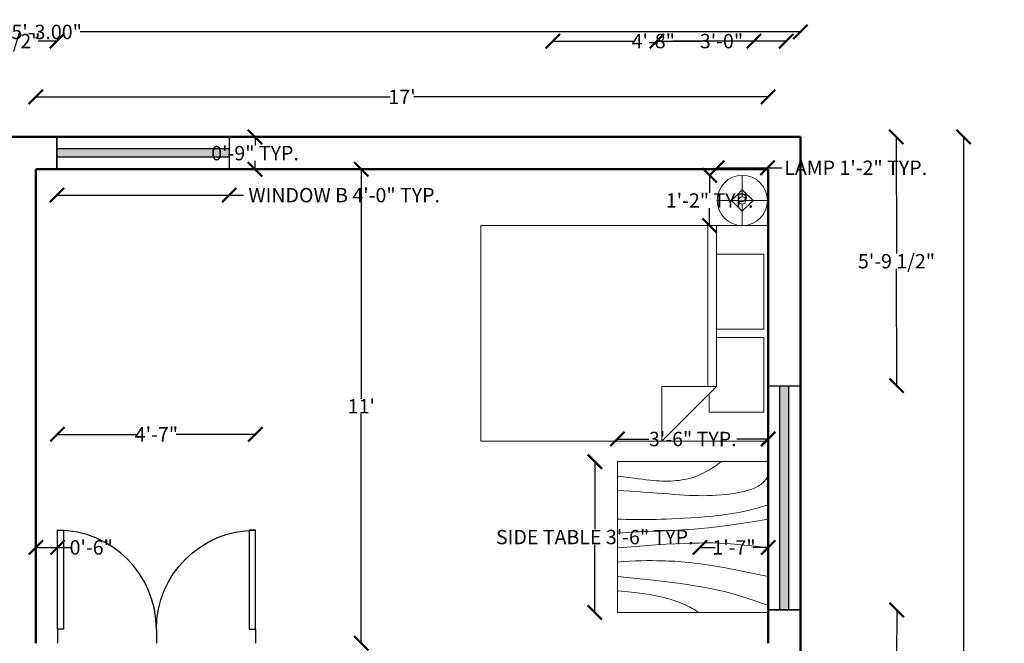
# Model space of a CAD drawing. Units: inches. Extents: x 2466 to 2986, y -30 to 527.
# Tile 5 of 5: x 2711 to 2986, y 354 to 527. Entities that reach past the tile are written whole.
import ezdxf

# ---------------------------------------------------------------- set-up
doc = ezdxf.new("R2010")
doc.units = ezdxf.units.IN
for name, color, linetype, lineweight in [('A-ANNO-DIMS', 2, 'Continuous', 18), ('A-GLAZ', 4, 'Continuous', 25), ('doors', 3, 'Continuous', 25), ('furniture', 6, 'Continuous', 18), ('walls', 40, 'Continuous', 50)]:
    doc.layers.add(name, color=color, linetype=linetype, lineweight=lineweight)
doc.styles.get("Standard").update_dxf_attribs({"font": 'arial.ttf'})
doc.dimstyles.get("Standard").update_dxf_attribs({"dimtxt": 4, "dimasz": 4, "dimexe": 0.18, "dimexo": 0.0625, "dimgap": 0.09, "dimtad": 0, "dimtih": 1, "dimtoh": 1, "dimzin": 0, "dimdsep": 46, "dimlunit": 3, "dimtxsty": 'Standard', "dimblk": 'ARCHTICK', "dimcen": 0.09, "dimse1": 1, "dimse2": 1, "dimclrd": 3, "dimclrt": 2, "dimadec": 0, "dimazin": 0, "dimtfac": 1, "dimtofl": 0, "dimtmove": 0, "dimatfit": 3, "dimfxl": 1, "dimtolj": 1, "dimtzin": 0, "dimarcsym": 0})

# ---------------------------------------------------------------- blocks, each defined once
blk = doc.blocks.new('*U8')
for p, q in [((0, 0), (0, -100)), ((700, 0), (700, -100))]:
    blk.add_line(p, q)
blk.add_lwpolyline([(0, 0), (0, 700), (43.75, 700), (43.75, 0)], close=True)
blk.add_arc((0, 0), 700, 0, 90)
blk = doc.blocks.new('Bed - Queen')
for p, q in [((0, -80.00003), (0, 0)), ((0, 0), (59.99999, 0)), ((59.99999, 0), (59.99999, -80.00003)), ((7.99999, -1.2), (28.79998, -1.2)), ((7.99999, -14.4), (7.99999, -1.2)), ((28.79998, -1.2), (28.79998, -14.4)), ((31.19999, -1.2), (51.99999, -1.2)), ((31.19999, -14.4), (31.19999, -1.2)), ((51.99999, -1.2), (51.99999, -16.4)), ((0, -14.4), (44.8, -14.4)), ((59.99999, -29.6), (44.8, -14.4)), ((44.8, -14.4), (44.8, -29.6)), ((51.99999, -16.4), (46.79936, -16.4)), ((44.8, -16.8), (0, -16.8)), ((44.8, -29.6), (59.99999, -29.6)), ((59.99999, -80.00003), (0, -80.00003))]:
    blk.add_line(p, q)
blk = doc.blocks.new('Lamp - Table')
for p, q in [((0, 7), (0, 1)), ((0, 3), (-3, 0)), ((3, 0), (0, 3)), ((-1, 0), (-7, 0)), ((-3, 0), (0, -3)), ((0, -3), (3, 0)), ((1, 0), (7, 0)), ((0, -1), (0, -7))]:
    blk.add_line(p, q)
for radius in [7, 1]:
    blk.add_circle((0, 0), radius)
blk = doc.blocks.new('Table - Square Woodgrain 42 x 42 in.')
blk.add_line((0, -42), (42, -42))
for points in [[(0, -4), (1.704, -4.2172), (3.2358, -4.4188), (4.615, -4.604), (5.8615, -4.7721), (6.9951, -4.9224), (8.0357, -5.0541), (9.0031, -5.1667), (9.9171, -5.2594), (10.7951, -5.3316), (11.6445, -5.3836), (12.4702, -5.4157), (13.277, -5.4283), (14.0698, -5.4217), (14.8535, -5.3964), (15.6331, -5.3526), (16.4133, -5.2908), (17.1986, -5.2103), (17.9913, -5.1062), (18.793, -4.9727), (19.6056, -4.8038), (20.4307, -4.5937), (21.2701, -4.3365), (22.1256, -4.0262), (22.9989, -3.6571), (23.888, -3.2272), (24.7756, -2.7516), (25.6408, -2.2491), (26.4624, -1.7387), (27.2195, -1.2395), (27.891, -0.7703), (28.456, -0.3501), (28.8934, 0.002)], [(0, -42), (0, 0), (42, 0), (42, -42)], [(0, -8), (1.8203, -8.1001), (3.6741, -8.2149), (5.5411, -8.3408), (7.4011, -8.4741), (9.2339, -8.6112), (11.0193, -8.7484), (12.7371, -8.8821), (14.3671, -9.0086), (15.8954, -9.1246), (17.3337, -9.2278), (18.6997, -9.3159), (20.0116, -9.387), (21.2871, -9.4389), (22.5442, -9.4696), (23.8008, -9.477), (25.0749, -9.459), (26.3791, -9.4137), (27.7049, -9.3403), (29.0383, -9.2382), (30.3655, -9.1068), (31.6728, -8.9455), (32.9461, -8.7535), (34.1717, -8.5304), (35.3358, -8.2756), (36.4268, -7.9863), (37.443, -7.6521), (38.3849, -7.2603), (39.253, -6.7986), (40.048, -6.2542), (40.7705, -5.6147), (41.421, -4.8674), (42, -4)], [(42, -12), (39.1784, -12.8621), (36.4519, -13.5654), (33.8246, -14.1294), (31.3004, -14.5731), (28.8832, -14.9161), (26.577, -15.1775), (24.3858, -15.3768), (22.3136, -15.5332), (20.3622, -15.6632), (18.5254, -15.7718), (16.7947, -15.8612), (15.1618, -15.9338), (13.6183, -15.9916), (12.1558, -16.0369), (10.7659, -16.0718), (9.4403, -16.0987), (8.1703, -16.1191), (6.9461, -16.1325), (5.7577, -16.1377), (4.595, -16.1335), (3.4479, -16.1188), (2.3064, -16.0924), (1.1604, -16.0532), (0, -16)], [(42, -16), (37.6529, -16.7365), (33.8802, -17.329), (30.6179, -17.7961), (27.8015, -18.1561), (25.3668, -18.4275), (23.2497, -18.6288), (21.3859, -18.7785), (19.7111, -18.8949), (18.1693, -18.9939), (16.7375, -19.0795), (15.401, -19.1534), (14.1449, -19.217), (12.9544, -19.2717), (11.8148, -19.3191), (10.7113, -19.3606), (9.6291, -19.3976), (8.5534, -19.4323), (7.47, -19.4689), (6.3643, -19.5122), (5.222, -19.5672), (4.0288, -19.6386), (2.7703, -19.7313), (1.4321, -19.8501), (0, -20)], [(0, -24), (3.9243, -23.6805), (7.4766, -23.4138), (10.6891, -23.1954), (13.5943, -23.0205), (16.2247, -22.8847), (18.6125, -22.7832), (20.7903, -22.7116), (22.7903, -22.6651), (24.6563, -22.642), (26.4764, -22.6507), (28.35, -22.7024), (30.3766, -22.8084), (32.6555, -22.98), (35.2861, -23.2283), (38.3678, -23.5645), (42, -24)], [(42, -32), (37.392, -31.017), (33.4585, -30.2231), (30.1291, -29.5949), (27.3334, -29.109), (25.0009, -28.742), (23.0612, -28.4707), (21.4439, -28.2716), (20.0786, -28.1215), (18.8998, -28.0002), (17.8609, -27.9014), (16.9206, -27.8219), (16.0371, -27.7588), (15.1691, -27.709), (14.2748, -27.6693), (13.3128, -27.6368), (12.2415, -27.6083), (11.0295, -27.5824), (9.6867, -27.5643), (8.233, -27.5608), (6.6884, -27.5787), (5.0728, -27.6248), (3.4062, -27.7058), (1.7086, -27.8286), (0, -28)], [(0, -32), (5.4026, -32.5358), (9.9494, -33.019), (13.7424, -33.4553), (16.8834, -33.8505), (19.4743, -34.2106), (21.6171, -34.5413), (23.4136, -34.8486), (24.9657, -35.1382), (26.3614, -35.4156), (27.6332, -35.6841), (28.7995, -35.9467), (29.8788, -36.2064), (30.8897, -36.4661), (31.8507, -36.7288), (32.7802, -36.9973), (33.6968, -37.2747), (34.6175, -37.5635), (35.5531, -37.8651), (36.5128, -38.1805), (37.506, -38.5108), (38.5421, -38.8568), (39.6302, -39.2197), (40.7797, -39.6004), (42, -40)], [(0, -36), (3.0098, -36.2857), (5.5354, -36.5643), (7.6368, -36.8359), (9.374, -37.1009), (10.807, -37.3597), (11.9957, -37.6126), (13.0002, -37.8599), (13.8804, -38.102), (14.6874, -38.3393), (15.4365, -38.5729), (16.1338, -38.8041), (16.7858, -39.0341), (17.3987, -39.264), (17.9787, -39.4952), (18.5322, -39.7288), (19.0655, -39.9662), (19.5832, -40.2081), (20.0842, -40.4544), (20.5657, -40.7046), (21.0249, -40.9581), (21.459, -41.2144), (21.8653, -41.4731), (22.2409, -41.7335), (22.5831, -41.9951)]]:
    blk.add_lwpolyline(points)
blk = doc.blocks.new('_ArchTick')
at = {"color": 0, "linetype": 'ByBlock', "const_width": 0.15}
blk.add_lwpolyline([(-0.5, -0.5), (0.5, 0.5)], dxfattribs=at)
blk = doc.blocks.new('*D21')
at = {"layer": 'A-ANNO-DIMS', "color": 0, "lineweight": -2, "transparency": 16777216}
for p, q in [((2505.73, 524.05), (2706.38, 524.05)), ((2928.73, 524.05), (2728.07, 524.05))]:
    blk.add_line(p, q, dxfattribs=at)
at = {"layer": 'Defpoints', "color": 0, "transparency": 16777216}
for p in [(2928.73, 524.05), (2505.73, 494.8), (2928.73, 494.8)]:
    blk.add_point(p, dxfattribs=at)
at = {"layer": 'A-ANNO-DIMS', "color": 0, "lineweight": -2, "transparency": 16777216, "xscale": 4, "yscale": 4, "zscale": 4, "rotation": 180}
blk.add_blockref('_ArchTick', (2505.73, 524.05), dxfattribs=at)
at = {"layer": 'A-ANNO-DIMS', "color": 0, "lineweight": -2, "transparency": 16777216, "xscale": 4, "yscale": 4, "zscale": 4}
blk.add_blockref('_ArchTick', (2928.73, 524.05), dxfattribs=at)
at = {"layer": 'A-ANNO-DIMS', "color": 0, "transparency": 16777216, "insert": (2717.23, 524.05), "char_height": 4, "attachment_point": 5}
blk.add_mtext('\\A1;35\'-3.00"', dxfattribs=at)
blk = doc.blocks.new('*D22')
at = {"layer": 'A-ANNO-DIMS', "color": 0, "lineweight": -2, "transparency": 16777216}
for p, q in [((2974.18, 494.8), (2974.18, 249.43)), ((2974.18, -0.2), (2974.18, 245.16))]:
    blk.add_line(p, q, dxfattribs=at)
at = {"layer": 'Defpoints', "color": 0, "transparency": 16777216}
for p in [(2928.73, 494.8), (2928.73, -0.2), (2974.18, -0.2)]:
    blk.add_point(p, dxfattribs=at)
at = {"layer": 'A-ANNO-DIMS', "color": 0, "lineweight": -2, "transparency": 16777216, "xscale": 4, "yscale": 4, "zscale": 4}
for p, rotation in [((2974.18, 494.8), 90), ((2974.18, -0.2), 270)]:
    blk.add_blockref('_ArchTick', p, dxfattribs=dict(at, rotation=rotation))
at = {"layer": 'A-ANNO-DIMS', "color": 0, "transparency": 16777216, "insert": (2974.18, 247.3), "char_height": 4, "attachment_point": 5}
blk.add_mtext('\\A1;41\'-3.00"', dxfattribs=at)
blk = doc.blocks.new('*D24')
at = {"layer": 'A-ANNO-DIMS', "color": 0, "lineweight": -2, "transparency": 16777216}
for p, q in [((2715.73, 505.95), (2814.43, 505.95)), ((2919.73, 505.95), (2821.02, 505.95))]:
    blk.add_line(p, q, dxfattribs=at)
at = {"layer": 'Defpoints', "color": 0, "transparency": 16777216}
for p in [(2919.73, 505.95), (2715.73, 485.8), (2919.73, 485.8)]:
    blk.add_point(p, dxfattribs=at)
at = {"layer": 'A-ANNO-DIMS', "color": 0, "lineweight": -2, "transparency": 16777216, "xscale": 4, "yscale": 4, "zscale": 4, "rotation": 180}
blk.add_blockref('_ArchTick', (2715.73, 505.95), dxfattribs=at)
at = {"layer": 'A-ANNO-DIMS', "color": 0, "lineweight": -2, "transparency": 16777216, "xscale": 4, "yscale": 4, "zscale": 4}
blk.add_blockref('_ArchTick', (2919.73, 505.95), dxfattribs=at)
at = {"layer": 'A-ANNO-DIMS', "color": 0, "transparency": 16777216, "insert": (2817.73, 505.95), "char_height": 4, "attachment_point": 5}
blk.add_mtext("\\A1;17'", dxfattribs=at)
blk = doc.blocks.new('*D26')
at = {"layer": 'A-ANNO-DIMS', "color": 0, "lineweight": -2, "transparency": 16777216}
for p, q in [((2806.39, 485.8), (2806.39, 421.89)), ((2806.39, 353.8), (2806.39, 417.7))]:
    blk.add_line(p, q, dxfattribs=at)
at = {"layer": 'Defpoints', "color": 0, "transparency": 16777216}
for p in [(2715.73, 485.8), (2715.73, 353.8), (2806.39, 353.8)]:
    blk.add_point(p, dxfattribs=at)
at = {"layer": 'A-ANNO-DIMS', "color": 0, "lineweight": -2, "transparency": 16777216, "xscale": 4, "yscale": 4, "zscale": 4}
for p, rotation in [((2806.39, 485.8), 90), ((2806.39, 353.8), 270)]:
    blk.add_blockref('_ArchTick', p, dxfattribs=dict(at, rotation=rotation))
at = {"layer": 'A-ANNO-DIMS', "color": 0, "transparency": 16777216, "insert": (2806.39, 419.8), "char_height": 4, "attachment_point": 5}
blk.add_mtext("\\A1;11'", dxfattribs=at)
blk = doc.blocks.new('WIN-62_38IN')
h = blk.add_hatch(color=256)
h.dxf.hatch_style = 1
h.paths.add_polyline_path([(3.19, 0), (5.61, 0), (5.61, 62.38), (3.19, 62.38)])
for p, q in [((0, 62.38), (9, 62.38)), ((0, 0), (9, 0))]:
    blk.add_line(p, q)
for points in [[(0, 0), (0, 62.38), (9, 62.38), (9, 62.38), (9, 0)], [(3.19, 0), (3.19, 62.38), (5.61, 62.38), (5.61, 0)]]:
    blk.add_lwpolyline(points, close=True)
blk = doc.blocks.new('WIN-48IN')
h = blk.add_hatch(color=256)
h.dxf.hatch_style = 1
h.paths.add_polyline_path([(0, 5.81), (0, 3.39), (48, 3.39), (48, 5.81)])
for p, q in [((0, 9), (0, 0)), ((48, 9), (48, 0))]:
    blk.add_line(p, q)
for points in [[(0, 9), (48, 9), (48, 0), (0, 0)], [(0, 5.81), (48, 5.81), (48, 3.39), (0, 3.39)]]:
    blk.add_lwpolyline(points, close=True)
blk = doc.blocks.new('*D41')
at = {"layer": 'A-ANNO-DIMS', "color": 3, "lineweight": -2, "transparency": 16777216}
for p, q in [((2721.59, 478.6), (2769.59, 478.6)), ((2769.59, 478.6), (2773.59, 478.6))]:
    blk.add_line(p, q, dxfattribs=at)
at = {"layer": 'Defpoints', "color": 0, "transparency": 16777216}
for p in [(2721.59, 485.8), (2769.59, 485.8), (2769.59, 478.6)]:
    blk.add_point(p, dxfattribs=at)
at = {"layer": 'A-ANNO-DIMS', "color": 3, "lineweight": -2, "transparency": 16777216, "xscale": 4, "yscale": 4, "zscale": 4, "rotation": 180}
blk.add_blockref('_ArchTick', (2721.59, 478.6), dxfattribs=at)
at = {"layer": 'A-ANNO-DIMS', "color": 3, "lineweight": -2, "transparency": 16777216, "xscale": 4, "yscale": 4, "zscale": 4}
blk.add_blockref('_ArchTick', (2769.59, 478.6), dxfattribs=at)
at = {"layer": 'A-ANNO-DIMS', "color": 2, "transparency": 16777216, "insert": (2801.63, 478.6), "char_height": 4, "attachment_point": 5}
blk.add_mtext('\\A1;WINDOW B 4\'-0" TYP.', dxfattribs=at)
blk = doc.blocks.new('*D42')
at = {"layer": 'A-ANNO-DIMS', "color": 3, "lineweight": -2, "transparency": 16777216}
for p, q in [((2776.79, 494.8), (2776.79, 492.43)), ((2776.79, 485.8), (2776.79, 488.16))]:
    blk.add_line(p, q, dxfattribs=at)
at = {"layer": 'Defpoints', "color": 0, "transparency": 16777216}
for p in [(2769.59, 494.8), (2776.79, 494.8), (2769.59, 485.8)]:
    blk.add_point(p, dxfattribs=at)
at = {"layer": 'A-ANNO-DIMS', "color": 3, "lineweight": -2, "transparency": 16777216, "xscale": 4, "yscale": 4, "zscale": 4}
for p, rotation in [((2776.79, 494.8), 90), ((2776.79, 485.8), 270)]:
    blk.add_blockref('_ArchTick', p, dxfattribs=dict(at, rotation=rotation))
at = {"layer": 'A-ANNO-DIMS', "color": 2, "transparency": 16777216, "insert": (2776.79, 490.3), "char_height": 4, "attachment_point": 5}
blk.add_mtext('\\A1;0\'-9" TYP.', dxfattribs=at)
blk = doc.blocks.new('*D45')
at = {"layer": 'A-ANNO-DIMS', "color": 3, "lineweight": -2, "transparency": 16777216}
for p, q in [((2905.53, 486.22), (2919.53, 486.22)), ((2919.53, 486.22), (2923.53, 486.22))]:
    blk.add_line(p, q, dxfattribs=at)
at = {"layer": 'Defpoints', "color": 0, "transparency": 16777216}
for p in [(2919.53, 486.22), (2905.53, 484.12), (2919.53, 484.12)]:
    blk.add_point(p, dxfattribs=at)
at = {"layer": 'A-ANNO-DIMS', "color": 3, "lineweight": -2, "transparency": 16777216, "xscale": 4, "yscale": 4, "zscale": 4, "rotation": 180}
blk.add_blockref('_ArchTick', (2905.53, 486.22), dxfattribs=at)
at = {"layer": 'A-ANNO-DIMS', "color": 3, "lineweight": -2, "transparency": 16777216, "xscale": 4, "yscale": 4, "zscale": 4}
blk.add_blockref('_ArchTick', (2919.53, 486.22), dxfattribs=at)
at = {"layer": 'A-ANNO-DIMS', "color": 2, "transparency": 16777216, "insert": (2944.1, 486.22), "char_height": 4, "attachment_point": 5}
blk.add_mtext('\\A1;LAMP 1\'-2" TYP.', dxfattribs=at)
blk = doc.blocks.new('*D46')
at = {"layer": 'A-ANNO-DIMS', "color": 3, "lineweight": -2, "transparency": 16777216}
for p, q in [((2903.43, 484.12), (2903.43, 479.22)), ((2903.43, 470.12), (2903.43, 475.02))]:
    blk.add_line(p, q, dxfattribs=at)
at = {"layer": 'Defpoints', "color": 0, "transparency": 16777216}
for p in [(2903.43, 484.12), (2905.53, 484.12), (2905.53, 470.12)]:
    blk.add_point(p, dxfattribs=at)
at = {"layer": 'A-ANNO-DIMS', "color": 3, "lineweight": -2, "transparency": 16777216, "xscale": 4, "yscale": 4, "zscale": 4}
for p, rotation in [((2903.43, 484.12), 90), ((2903.43, 470.12), 270)]:
    blk.add_blockref('_ArchTick', p, dxfattribs=dict(at, rotation=rotation))
at = {"layer": 'A-ANNO-DIMS', "color": 2, "transparency": 16777216, "insert": (2903.43, 477.12), "char_height": 4, "attachment_point": 5}
blk.add_mtext('\\A1;1\'-2" TYP.', dxfattribs=at)
blk = doc.blocks.new('*D47')
at = {"layer": 'A-ANNO-DIMS', "color": 3, "lineweight": -2, "transparency": 16777216}
for p, q in [((2871.43, 404.39), (2871.43, 385.54)), ((2871.43, 362.38), (2871.43, 381.22))]:
    blk.add_line(p, q, dxfattribs=at)
at = {"layer": 'Defpoints', "color": 0, "transparency": 16777216}
for p in [(2871.43, 404.39), (2877.73, 404.39), (2877.73, 362.38)]:
    blk.add_point(p, dxfattribs=at)
at = {"layer": 'A-ANNO-DIMS', "color": 3, "lineweight": -2, "transparency": 16777216, "xscale": 4, "yscale": 4, "zscale": 4}
for p, rotation in [((2871.43, 404.39), 90), ((2871.43, 362.38), 270)]:
    blk.add_blockref('_ArchTick', p, dxfattribs=dict(at, rotation=rotation))
at = {"layer": 'A-ANNO-DIMS', "color": 2, "transparency": 16777216, "insert": (2871.43, 383.38), "char_height": 4, "attachment_point": 5}
blk.add_mtext('\\A1;SIDE TABLE 3\'-6" TYP.', dxfattribs=at)
blk = doc.blocks.new('*D48')
at = {"layer": 'A-ANNO-DIMS', "color": 3, "lineweight": -2, "transparency": 16777216}
for p, q in [((2877.73, 410.69), (2886.45, 410.69)), ((2919.73, 410.69), (2911.01, 410.69))]:
    blk.add_line(p, q, dxfattribs=at)
at = {"layer": 'Defpoints', "color": 0, "transparency": 16777216}
for p in [(2919.73, 410.69), (2877.73, 404.39), (2919.73, 404.39)]:
    blk.add_point(p, dxfattribs=at)
at = {"layer": 'A-ANNO-DIMS', "color": 3, "lineweight": -2, "transparency": 16777216, "xscale": 4, "yscale": 4, "zscale": 4, "rotation": 180}
blk.add_blockref('_ArchTick', (2877.73, 410.69), dxfattribs=at)
at = {"layer": 'A-ANNO-DIMS', "color": 3, "lineweight": -2, "transparency": 16777216, "xscale": 4, "yscale": 4, "zscale": 4}
blk.add_blockref('_ArchTick', (2919.73, 410.69), dxfattribs=at)
at = {"layer": 'A-ANNO-DIMS', "color": 2, "transparency": 16777216, "insert": (2898.73, 410.69), "char_height": 4, "attachment_point": 5}
blk.add_mtext('\\A1;3\'-6" TYP.', dxfattribs=at)
blk = doc.blocks.new('*D63')
at = {"layer": 'A-ANNO-DIMS', "color": 3, "lineweight": -2, "transparency": 16777216}
for p, q in [((2721.75, 411.99), (2743.83, 411.99)), ((2776.87, 411.99), (2754.8, 411.99))]:
    blk.add_line(p, q, dxfattribs=at)
at = {"layer": 'Defpoints', "color": 0, "transparency": 16777216}
for p in [(2776.87, 411.99), (2721.75, 385.29), (2776.87, 385.29)]:
    blk.add_point(p, dxfattribs=at)
at = {"layer": 'A-ANNO-DIMS', "color": 3, "lineweight": -2, "transparency": 16777216, "xscale": 4, "yscale": 4, "zscale": 4, "rotation": 180}
blk.add_blockref('_ArchTick', (2721.75, 411.99), dxfattribs=at)
at = {"layer": 'A-ANNO-DIMS', "color": 3, "lineweight": -2, "transparency": 16777216, "xscale": 4, "yscale": 4, "zscale": 4}
blk.add_blockref('_ArchTick', (2776.87, 411.99), dxfattribs=at)
at = {"layer": 'A-ANNO-DIMS', "color": 2, "transparency": 16777216, "insert": (2749.31, 411.99), "char_height": 4, "attachment_point": 5}
blk.add_mtext('\\A1;4\'-7"', dxfattribs=at)
blk = doc.blocks.new('*D67')
at = {"layer": 'A-ANNO-DIMS', "color": 3, "lineweight": -2, "transparency": 16777216}
for p, q in [((2888.73, 521.5), (2901.32, 521.5)), ((2924.73, 521.5), (2912.13, 521.5))]:
    blk.add_line(p, q, dxfattribs=at)
at = {"layer": 'Defpoints', "color": 0, "transparency": 16777216}
for p in [(2924.73, 521.5), (2888.73, 47.8), (2924.73, 47.8)]:
    blk.add_point(p, dxfattribs=at)
at = {"layer": 'A-ANNO-DIMS', "color": 3, "lineweight": -2, "transparency": 16777216, "xscale": 4, "yscale": 4, "zscale": 4, "rotation": 180}
blk.add_blockref('_ArchTick', (2888.73, 521.5), dxfattribs=at)
at = {"layer": 'A-ANNO-DIMS', "color": 3, "lineweight": -2, "transparency": 16777216, "xscale": 4, "yscale": 4, "zscale": 4}
blk.add_blockref('_ArchTick', (2924.73, 521.5), dxfattribs=at)
at = {"layer": 'A-ANNO-DIMS', "color": 2, "transparency": 16777216, "insert": (2906.73, 521.5), "char_height": 4, "attachment_point": 5}
blk.add_mtext('\\A1;3\'-0"', dxfattribs=at)
blk = doc.blocks.new('*D70')
at = {"layer": 'A-ANNO-DIMS', "color": 3, "lineweight": -2, "transparency": 16777216}
for p, q in [((2859.73, 521.5), (2882.24, 521.5)), ((2915.73, 521.5), (2893.21, 521.5))]:
    blk.add_line(p, q, dxfattribs=at)
at = {"layer": 'Defpoints', "color": 0, "transparency": 16777216}
for p in [(2915.73, 521.5), (2859.73, 140.8), (2915.73, 140.8)]:
    blk.add_point(p, dxfattribs=at)
at = {"layer": 'A-ANNO-DIMS', "color": 3, "lineweight": -2, "transparency": 16777216, "xscale": 4, "yscale": 4, "zscale": 4, "rotation": 180}
blk.add_blockref('_ArchTick', (2859.73, 521.5), dxfattribs=at)
at = {"layer": 'A-ANNO-DIMS', "color": 3, "lineweight": -2, "transparency": 16777216, "xscale": 4, "yscale": 4, "zscale": 4}
blk.add_blockref('_ArchTick', (2915.73, 521.5), dxfattribs=at)
at = {"layer": 'A-ANNO-DIMS', "color": 2, "transparency": 16777216, "insert": (2887.73, 521.5), "char_height": 4, "attachment_point": 5}
blk.add_mtext('\\A1;4\'-8"', dxfattribs=at)
blk = doc.blocks.new('*D73')
at = {"layer": 'A-ANNO-DIMS', "color": 3, "lineweight": -2, "transparency": 16777216}
for p, q in [((2690.98, 521.5), (2696.18, 521.5)), ((2721.59, 521.5), (2716.38, 521.5))]:
    blk.add_line(p, q, dxfattribs=at)
at = {"layer": 'Defpoints', "color": 0, "transparency": 16777216}
for p in [(2721.59, 521.5), (2690.98, 494.8), (2721.59, 494.8)]:
    blk.add_point(p, dxfattribs=at)
at = {"layer": 'A-ANNO-DIMS', "color": 3, "lineweight": -2, "transparency": 16777216, "xscale": 4, "yscale": 4, "zscale": 4, "rotation": 180}
blk.add_blockref('_ArchTick', (2690.98, 521.5), dxfattribs=at)
at = {"layer": 'A-ANNO-DIMS', "color": 3, "lineweight": -2, "transparency": 16777216, "xscale": 4, "yscale": 4, "zscale": 4}
blk.add_blockref('_ArchTick', (2721.59, 521.5), dxfattribs=at)
at = {"layer": 'A-ANNO-DIMS', "color": 2, "transparency": 16777216, "insert": (2706.28, 521.5), "char_height": 4, "attachment_point": 5}
blk.add_mtext('\\A1;2\'-6 1/2"', dxfattribs=at)
blk = doc.blocks.new('*D77')
at = {"layer": 'A-ANNO-DIMS', "color": 3, "lineweight": -2, "transparency": 16777216}
for p, q in [((2955.43, 494.83), (2955.47, 462.36)), ((2955.53, 425.57), (2955.48, 458.05))]:
    blk.add_line(p, q, dxfattribs=at)
at = {"layer": 'Defpoints', "color": 0, "transparency": 16777216}
for p in [(2928.73, 494.8), (2928.83, 425.53), (2955.53, 425.57)]:
    blk.add_point(p, dxfattribs=at)
at = {"layer": 'A-ANNO-DIMS', "color": 3, "lineweight": -2, "transparency": 16777216, "xscale": 4, "yscale": 4, "zscale": 4}
for p, rotation in [((2955.43, 494.83), 90.08446035747114), ((2955.53, 425.57), 270.0844603574712)]:
    blk.add_blockref('_ArchTick', p, dxfattribs=dict(at, rotation=rotation))
at = {"layer": 'A-ANNO-DIMS', "color": 2, "transparency": 16777216, "insert": (2955.48, 460.2), "char_height": 4, "attachment_point": 5}
blk.add_mtext('\\A1;5\'-9 1/2"', dxfattribs=at)
blk = doc.blocks.new('*D83')
at = {"layer": 'A-ANNO-DIMS', "color": 3, "lineweight": -2, "transparency": 16777216}
for p, q in [((2955.53, 363.07), (2955.48, 349.01)), ((2955.43, 330.64), (2955.47, 344.7))]:
    blk.add_line(p, q, dxfattribs=at)
at = {"layer": 'Defpoints', "color": 0, "transparency": 16777216}
for p in [(2928.83, 363.15), (2928.73, 330.72), (2955.43, 330.64)]:
    blk.add_point(p, dxfattribs=at)
at = {"layer": 'A-ANNO-DIMS', "color": 3, "lineweight": -2, "transparency": 16777216, "xscale": 4, "yscale": 4, "zscale": 4}
for p, rotation in [((2955.53, 363.07), 89.81962137861794), ((2955.43, 330.64), 269.8196213786179)]:
    blk.add_blockref('_ArchTick', p, dxfattribs=dict(at, rotation=rotation))
at = {"layer": 'A-ANNO-DIMS', "color": 2, "transparency": 16777216, "insert": (2955.48, 346.85), "char_height": 4, "attachment_point": 5}
blk.add_mtext('\\A1;2\'-8 1/2"', dxfattribs=at)
blk = doc.blocks.new('*D86')
at = {"layer": 'A-ANNO-DIMS', "color": 3, "lineweight": -2, "transparency": 16777216}
for p, q in [((2715.73, 380.5), (2721.75, 380.5)), ((2721.75, 380.5), (2725.75, 380.5))]:
    blk.add_line(p, q, dxfattribs=at)
at = {"layer": 'Defpoints', "color": 0, "transparency": 16777216}
for p in [(2721.75, 380.5), (2715.73, 353.8), (2721.75, 353.8)]:
    blk.add_point(p, dxfattribs=at)
at = {"layer": 'A-ANNO-DIMS', "color": 3, "lineweight": -2, "transparency": 16777216, "xscale": 4, "yscale": 4, "zscale": 4, "rotation": 180}
blk.add_blockref('_ArchTick', (2715.73, 380.5), dxfattribs=at)
at = {"layer": 'A-ANNO-DIMS', "color": 3, "lineweight": -2, "transparency": 16777216, "xscale": 4, "yscale": 4, "zscale": 4}
blk.add_blockref('_ArchTick', (2721.75, 380.5), dxfattribs=at)
at = {"layer": 'A-ANNO-DIMS', "color": 2, "transparency": 16777216, "insert": (2731.16, 380.5), "char_height": 4, "attachment_point": 5}
blk.add_mtext('\\A1;0\'-6"', dxfattribs=at)
blk = doc.blocks.new('*D87')
at = {"layer": 'A-ANNO-DIMS', "color": 3, "lineweight": -2, "transparency": 16777216}
for p, q in [((2900.7, 380.5), (2904.99, 380.5)), ((2919.73, 380.5), (2915.43, 380.5))]:
    blk.add_line(p, q, dxfattribs=at)
at = {"layer": 'Defpoints', "color": 0, "transparency": 16777216}
for p in [(2919.73, 380.5), (2900.7, 353.8), (2919.73, 353.8)]:
    blk.add_point(p, dxfattribs=at)
at = {"layer": 'A-ANNO-DIMS', "color": 3, "lineweight": -2, "transparency": 16777216, "xscale": 4, "yscale": 4, "zscale": 4, "rotation": 180}
blk.add_blockref('_ArchTick', (2900.7, 380.5), dxfattribs=at)
at = {"layer": 'A-ANNO-DIMS', "color": 3, "lineweight": -2, "transparency": 16777216, "xscale": 4, "yscale": 4, "zscale": 4}
blk.add_blockref('_ArchTick', (2919.73, 380.5), dxfattribs=at)
at = {"layer": 'A-ANNO-DIMS', "color": 2, "transparency": 16777216, "insert": (2910.21, 380.5), "char_height": 4, "attachment_point": 5}
blk.add_mtext('\\A1;1\'-7"', dxfattribs=at)

msp = doc.modelspace()

# ---------------------------------------------------------------- linework, layer by layer
at = {"layer": 'walls'}
for p, q in [((2690.976, 494.795), (2928.725, 494.795)), ((2928.725, 494.795), (2928.725, 131.795)), ((2715.725, 485.795), (2715.725, 353.795)), ((2715.725, 485.795), (2919.725, 485.795)), ((2919.725, 485.795), (2919.725, 353.795))]:
    msp.add_line(p, q, dxfattribs=at)

# ---------------------------------------------------------------- block references
at = {"layer": 'A-GLAZ'}
for name, p in [('WIN-48IN', (2721.59, 485.795)), ('WIN-62_38IN', (2919.828, 363.154))]:
    msp.add_blockref(name, p, dxfattribs=at)
at = {"layer": 'doors', "yscale": 0.0393700787401575, "zscale": 0.0393700787401575}
for p, xscale in [((2721.753, 357.732), 0.0393700787401575), ((2776.871, 357.732), -0.0393700787401575)]:
    msp.add_blockref('*U8', p, dxfattribs=dict(at, xscale=xscale))
at = {"layer": 'furniture'}
for name, p in [('Lamp - Table', (2912.525, 477.118)), ('Table - Square Woodgrain 42 x 42 in.', (2877.725, 404.383))]:
    msp.add_blockref(name, p, dxfattribs=at)
at = {"layer": 'furniture', "rotation": 270}
msp.add_blockref('Bed - Queen', (2919.725, 470.118), dxfattribs=at)

# ---------------------------------------------------------------- dimensions: what is measured, and where the dimension line sits
at = {"layer": 'A-ANNO-DIMS'}
for base, p1, p2, override, picture, middle in [((2928.725, 524.047), (2505.725, 494.795), (2928.725, 494.795), {"dimclrd": 0, "dimclre": 0, "dimclrt": 0}, '*D21', (2717.225, 524.047)), ((2721.59, 521.495), (2690.976, 494.795), (2721.59, 494.795), {"dimdec": 1, "dimlfac": 1, "dimrnd": 0, "dimzin": 1, "dimdsep": 46, "dimlunit": 4, "dimfrac": 2}, '*D73', (2706.283, 521.495)), ((2915.725, 521.495), (2859.725, 140.795), (2915.725, 140.795), {"dimdec": 1, "dimlfac": 1, "dimrnd": 0, "dimzin": 1, "dimdsep": 46, "dimlunit": 4, "dimfrac": 2}, '*D70', (2887.725, 521.495)), ((2924.725, 521.495), (2888.725, 47.795), (2924.725, 47.795), {"dimdec": 1, "dimlfac": 1, "dimrnd": 0, "dimzin": 1, "dimdsep": 46, "dimlunit": 4, "dimfrac": 2}, '*D67', (2906.725, 521.495)), ((2919.725, 505.95), (2715.725, 485.795), (2919.725, 485.795), {"dimclrd": 0, "dimclre": 0, "dimclrt": 0}, '*D24', (2817.725, 505.95)), ((2776.871, 411.992), (2721.753, 385.292), (2776.871, 385.292), {"dimdec": 1, "dimlfac": 1, "dimrnd": 0, "dimzin": 1, "dimdsep": 46, "dimlunit": 4, "dimfrac": 2}, '*D63', (2749.312, 411.992)), ((2721.753, 380.495), (2715.725, 353.795), (2721.753, 353.795), {"dimdec": 1, "dimlfac": 1, "dimrnd": 0, "dimzin": 1, "dimdsep": 46, "dimlunit": 4, "dimfrac": 2}, '*D86', (2731.16, 380.495)), ((2919.725, 380.495), (2900.701, 353.795), (2919.725, 353.795), {"dimdec": 1, "dimlfac": 1, "dimrnd": 0, "dimzin": 1, "dimdsep": 46, "dimlunit": 4, "dimfrac": 2}, '*D87', (2910.213, 380.495))]:
    dim = msp.add_linear_dim(base=base, p1=p1, p2=p2, dimstyle='Standard', override=override, dxfattribs=at)
    dim.commit()
    dim.dimension.update_dxf_attribs({"geometry": picture, "text_midpoint": middle})
for base, p1, p2, text, picture, middle in [((2776.79, 494.795), (2769.59, 485.795), (2769.59, 494.795), '<> TYP.', '*D42', (2776.79, 490.295)), ((2903.425, 484.118), (2905.525, 470.118), (2905.525, 484.118), '<> TYP.', '*D46', (2903.425, 477.118)), ((2871.425, 404.385), (2877.725, 362.383), (2877.725, 404.385), 'SIDE TABLE <> TYP.', '*D47', (2871.425, 383.384))]:
    dim = msp.add_linear_dim(base=base, p1=p1, p2=p2, angle=90, text=text, dimstyle='Standard', override={"dimdec": 1, "dimlfac": 1, "dimrnd": 0, "dimzin": 1, "dimdsep": 46, "dimlunit": 4, "dimfrac": 2}, dxfattribs=at)
    dim.commit()
    dim.dimension.update_dxf_attribs({"geometry": picture, "text_midpoint": middle})
for base, p1, p2, angle, override, picture, middle in [((2955.528, 425.572), (2928.725, 494.795), (2928.828, 425.533), 270.08446, {"dimdec": 1, "dimlfac": 1, "dimrnd": 0, "dimzin": 1, "dimdsep": 46, "dimlunit": 4, "dimfrac": 2}, '*D77', (2955.477, 460.204)), ((2974.184, -0.205), (2928.725, 494.795), (2928.725, -0.205), 90, {"dimclrd": 0, "dimclre": 0, "dimclrt": 0}, '*D22', (2974.184, 247.295)), ((2806.394, 353.795), (2715.725, 485.795), (2715.725, 353.795), 90, {"dimclrd": 0, "dimclre": 0, "dimclrt": 0}, '*D26', (2806.394, 419.795)), ((2955.425, 330.639), (2928.828, 363.154), (2928.725, 330.723), 269.81962, {"dimdec": 1, "dimlfac": 1, "dimrnd": 0, "dimzin": 1, "dimdsep": 46, "dimlunit": 4, "dimfrac": 2}, '*D83', (2955.476, 346.854))]:
    dim = msp.add_linear_dim(base=base, p1=p1, p2=p2, angle=angle, dimstyle='Standard', override=override, dxfattribs=at)
    dim.commit()
    dim.dimension.update_dxf_attribs({"geometry": picture, "text_midpoint": middle})
for base, p1, p2, text, picture, middle in [((2919.525, 486.218), (2905.525, 484.118), (2919.525, 484.118), 'LAMP <> TYP.', '*D45', (2944.103, 486.218)), ((2769.59, 478.595), (2721.59, 485.795), (2769.59, 485.795), 'WINDOW B <> TYP.', '*D41', (2801.628, 478.595)), ((2919.725, 410.686), (2877.725, 404.385), (2919.725, 404.385), '<> TYP.', '*D48', (2898.725, 410.686))]:
    dim = msp.add_linear_dim(base=base, p1=p1, p2=p2, text=text, dimstyle='Standard', override={"dimdec": 1, "dimlfac": 1, "dimrnd": 0, "dimzin": 1, "dimdsep": 46, "dimlunit": 4, "dimfrac": 2}, dxfattribs=at)
    dim.commit()
    dim.dimension.update_dxf_attribs({"geometry": picture, "text_midpoint": middle})

doc.saveas('drawing.dxf')
